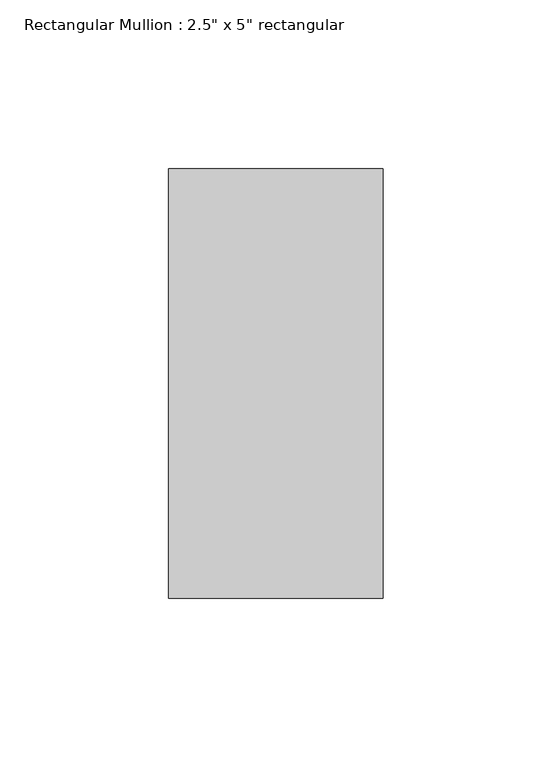
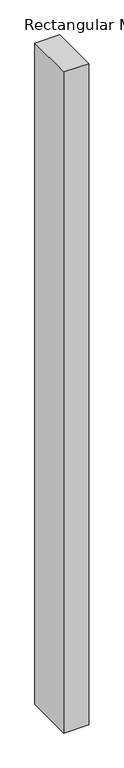
"""IFC4 building model written with IfcOpenShell, lengths in millimetres: member geometry."""

from ifc_helpers import new_model, si_unit, frame, origin, place, context, project, spatial, polyline, outline, extrude, source, transform, mapped, element, save


def member_e710c4d8(model_context):
    return source(origin(), model_context, "Body", "SweptSolid", [
        extrude(outline(polyline([(31.75, 63.5), (31.75, -63.5), (-31.75, -63.5), (-31.75, 63.5), (31.75, 63.5)])), frame((0.0, 0.0, -1777.3307027), z_axis=(0.0, 0.0, 1.0), x_axis=(1.0, 0.0, 0.0)), (0.0, 0.0, 1.0), 1777.3307027),
    ])


if __name__ == "__main__":
    model = new_model("IFC4")
    model_context = context("Model", 3, world=origin())
    ifc_project = project(units=[si_unit("LENGTHUNIT", "METRE", prefix="MILLI")], contexts=[model_context])
    site = spatial("IfcSite", under=ifc_project)
    building = spatial("IfcBuilding", under=site)
    placement = place(None, origin())
    member_shape = member_e710c4d8(model_context)
    element("IfcMember", 1, ObjectType="Rectangular Mullion : 2.5\" x 5\" rectangular", at=placement, inside=building, context=model_context, shape_type="MappedRepresentation", body=[
        mapped(member_shape, transform((0.0, 0.0, 0.0), x_axis=(1.0, 0.0, 0.0), y_axis=(0.0, 1.0, 0.0), z_axis=(0.0, 0.0, 1.0))),
    ])
    save(model, "model.ifc")

# Revit data of these elements
# Type "Rectangular Mullion : 2.5\" x 5\" rectangular"
#   built-in parameter 1007304 = 0.416667 (stored number, unit not read)
#   built-in parameter 1007301 = 0.104167 (stored number, unit not read)
#   built-in parameter 1007300 = 0.104167 (stored number, unit not read)
# Element 1 (IfcMember, "Rectangular Mullion : 2.5\" x 5\" rectangular")
#   Materials on its faces: "Aluminum"
# Materials
#   "Aluminum": class "Metal", colour RGB 247 247 247, transparency 0, Description = "Aluminum 6061", Cost = 0
